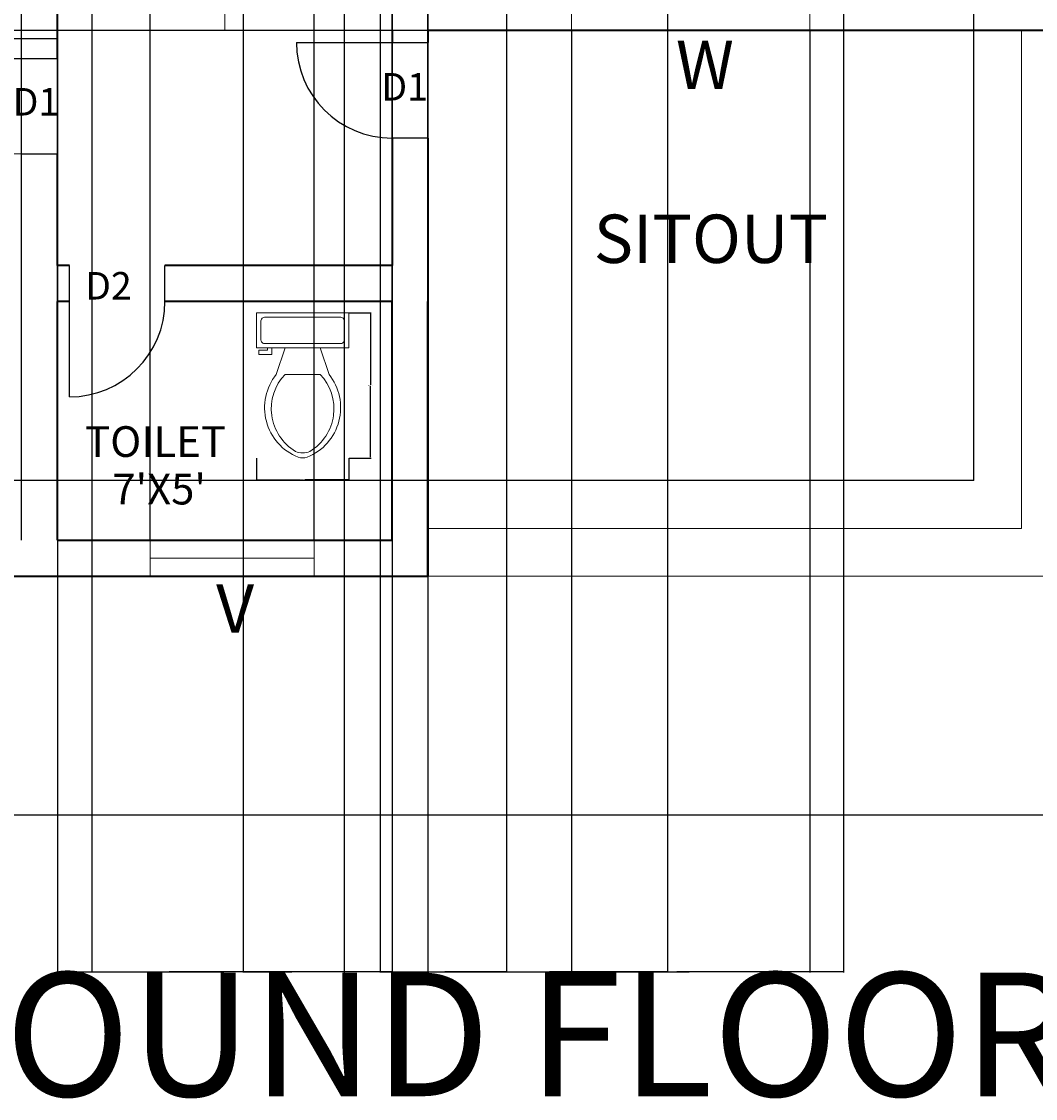
# Model space of a CAD drawing. Units: feet. Extents: x 2270 to 3094, y 1543 to 2352.
# Tile 2 of 6: x 2563 to 2817, y 1543 to 1813. Entities that reach past the tile are written whole.
import ezdxf

# ---------------------------------------------------------------- set-up
doc = ezdxf.new("R2010")
doc.units = ezdxf.units.FT
for name, color, linetype, lineweight in [('A-ANNO-DIMS', 2, 'Continuous', 18), ('A-ANNO-TEXT', 7, 'Continuous', 18), ('A-ANNO-TITL', 7, 'Continuous', 35), ('A-AREA-IDEN', 7, 'Continuous', 18), ('A-DOOR', 3, 'Continuous', 25), ('A-FLOR-FIXT', 8, 'Continuous', 18), ('A-FLOR-STRS', 7, 'Continuous', 18), ('A-GLAZ', 4, 'Continuous', 18), ('A-WALL', 7, 'Continuous', 35), ('C-PROP', 8, 'Continuous', 25)]:
    doc.layers.add(name, color=color, linetype=linetype, lineweight=lineweight)
doc.styles.get("Standard").update_dxf_attribs({"font": 'arial.ttf'})
doc.dimstyles.get("Standard").update_dxf_attribs({"dimtxt": 0.18, "dimasz": 0.18, "dimexe": 0.18, "dimexo": 0.0625, "dimgap": 0.09, "dimtad": 0, "dimtih": 1, "dimtoh": 1, "dimdec": 4, "dimzin": 0, "dimdsep": 46, "dimtxsty": 'Standard', "dimcen": 0.09, "dimadec": 0, "dimazin": 0, "dimtfac": 1, "dimtdec": 4, "dimtofl": 0, "dimtmove": 0, "dimatfit": 3, "dimfxl": 1, "dimtolj": 1, "dimtzin": 0, "dimarcsym": 0})

# ---------------------------------------------------------------- blocks, each defined once
blk = doc.blocks.new('Toilet - top')
for p, q in [((9.5, -6), (9.5, -2)), ((-10, -8.5), (-8, -8.5)), ((-10, -9.5), (-10, -8.5)), ((-7, -9.5), (-10, -9.5)), ((-8, -8.5), (-8, -8)), ((-7, -8), (-7, -9.5)), ((-4, -8), (-6, -14)), ((4, -8), (6, -14)), ((4, -14), (-4, -14))]:
    blk.add_line(p, q)
blk.add_lwpolyline([(10.5, -8), (10.5, 0), (-10.5, 0), (-10.5, -8)], close=True)
for points in [[(-9.5, -2), (-9.5, -6)], [(8.5, -1), (-8.5, -1)], [(-8.5, -7), (8.5, -7)]]:
    blk.add_lwpolyline(points)
for centre, radius, start, end in [((-8.62, -1.88), 0.884, 81.8699, 188.1301), ((8.62, -1.88), 0.884, 351.8699, 98.1301), ((-8.62, -6.12), 0.884, 171.8699, 278.1301), ((8.62, -6.12), 0.884, 261.8699, 8.1301), ((3.52, -21.58), 12.17, 141.4691, 247.9714), ((4.2, -21.82), 11.33, 136.3677, 238.9468), ((-3.52, -21.58), 12.17, 292.0284, 38.5307), ((-4.2, -21.82), 11.33, 301.053, 43.6321), ((0, -27.88), 4, 245.7318, 294.2682), ((0, -29), 4, 254.8605, 285.1395)]:
    blk.add_arc(centre, radius, start, end)
blk = doc.blocks.new('DOOR-SWING-24')
blk.add_line((33, 0), (0, 0))
blk.add_arc((9, 0), 24, 0, 90)
blk = doc.blocks.new('*D10')
at = {"layer": 'A-ANNO-DIMS', "color": 0, "lineweight": -2, "transparency": 16777216}
for p, q in [((2538.67, 1804.15), (2538.67, 1809.21)), ((2538.85, 1809.03), (2554.23, 1809.03)), ((2571.49, 1809.03), (2556.1, 1809.03)), ((2571.67, 1804.15), (2571.67, 1809.21))]:
    blk.add_line(p, q, dxfattribs=at)
at = {"layer": 'A-ANNO-DIMS', "color": 0, "transparency": 16777216}
for points in [[(2538.85, 1809.06), (2538.85, 1809), (2538.67, 1809.03)], [(2571.49, 1809.06), (2571.49, 1809), (2571.67, 1809.03)]]:
    blk.add_solid(points, dxfattribs=at)
at = {"layer": 'Defpoints', "color": 0, "transparency": 16777216}
for p in [(2538.67, 1809.03), (2538.67, 1804.08), (2571.67, 1804.08)]:
    blk.add_point(p, dxfattribs=at)
at = {"layer": 'A-ANNO-DIMS', "color": 0, "transparency": 16777216, "insert": (2555.17, 1809.03), "char_height": 0.18, "attachment_point": 5}
blk.add_mtext('\\A1;DOOR 33 TYP.', dxfattribs=at)
blk = doc.blocks.new('*D14')
at = {"layer": 'A-ANNO-DIMS', "color": 0, "lineweight": -2, "transparency": 16777216}
for p, q in [((2644.87, 1740.2), (2650.46, 1740.2)), ((2650.28, 1740.02), (2650.28, 1722.15)), ((2650.28, 1703.92), (2650.28, 1721.79)), ((2644.87, 1703.74), (2650.46, 1703.74))]:
    blk.add_line(p, q, dxfattribs=at)
at = {"layer": 'A-ANNO-DIMS', "color": 0, "transparency": 16777216}
for points in [[(2650.25, 1740.02), (2650.31, 1740.02), (2650.28, 1740.2)], [(2650.25, 1703.92), (2650.31, 1703.92), (2650.28, 1703.74)]]:
    blk.add_solid(points, dxfattribs=at)
at = {"layer": 'Defpoints', "color": 0, "transparency": 16777216}
for p in [(2644.81, 1740.2), (2650.28, 1740.2), (2644.81, 1703.74)]:
    blk.add_point(p, dxfattribs=at)
at = {"layer": 'A-ANNO-DIMS', "color": 0, "transparency": 16777216, "insert": (2650.28, 1721.97), "char_height": 0.18, "attachment_point": 5}
blk.add_mtext('\\A1;WC 36 TYP.', dxfattribs=at)
blk = doc.blocks.new('*D15')
at = {"layer": 'A-ANNO-DIMS', "color": 0, "lineweight": -2, "transparency": 16777216}
for p, q in [((2621.64, 1703.68), (2621.64, 1698.09)), ((2644.81, 1703.68), (2644.81, 1698.09)), ((2621.82, 1698.27), (2632.7, 1698.27)), ((2644.63, 1698.27), (2633.75, 1698.27))]:
    blk.add_line(p, q, dxfattribs=at)
at = {"layer": 'A-ANNO-DIMS', "color": 0, "transparency": 16777216}
for points in [[(2621.82, 1698.3), (2621.82, 1698.24), (2621.64, 1698.27)], [(2644.63, 1698.3), (2644.63, 1698.24), (2644.81, 1698.27)]]:
    blk.add_solid(points, dxfattribs=at)
at = {"layer": 'Defpoints', "color": 0, "transparency": 16777216}
for p in [(2621.64, 1703.74), (2644.81, 1703.74), (2644.81, 1698.27)]:
    blk.add_point(p, dxfattribs=at)
at = {"layer": 'A-ANNO-DIMS', "color": 0, "transparency": 16777216, "insert": (2633.23, 1698.27), "char_height": 0.18, "attachment_point": 5}
blk.add_mtext('\\A1;23 TYP.', dxfattribs=at)
blk = doc.blocks.new('*D34')
at = {"layer": 'A-ANNO-DIMS', "color": 0, "lineweight": -2, "transparency": 16777216}
for p, q in [((2580.32, 2252.02), (2580.32, 1574.6)), ((2618.3, 2252.02), (2618.3, 1574.6)), ((2580.5, 1574.78), (2598.92, 1574.78)), ((2618.12, 1574.78), (2599.7, 1574.78))]:
    blk.add_line(p, q, dxfattribs=at)
at = {"layer": 'A-ANNO-DIMS', "color": 0, "transparency": 16777216}
for points in [[(2580.5, 1574.81), (2580.5, 1574.75), (2580.32, 1574.78)], [(2618.12, 1574.81), (2618.12, 1574.75), (2618.3, 1574.78)]]:
    blk.add_solid(points, dxfattribs=at)
at = {"layer": 'Defpoints', "color": 0, "transparency": 16777216}
for p in [(2580.32, 2252.08), (2618.3, 2252.08), (2618.3, 1574.78)]:
    blk.add_point(p, dxfattribs=at)
at = {"layer": 'A-ANNO-DIMS', "color": 0, "transparency": 16777216, "insert": (2599.31, 1574.78), "char_height": 0.18, "attachment_point": 5}
blk.add_mtext('\\A1;37.98', dxfattribs=at)
blk = doc.blocks.new('*D35')
at = {"layer": 'A-ANNO-DIMS', "color": 0, "lineweight": -2, "transparency": 16777216}
for p, q in [((2618.3, 2243.02), (2618.3, 1574.6)), ((2643.67, 2243.02), (2643.67, 1574.6)), ((2618.48, 1574.78), (2630.52, 1574.78)), ((2643.49, 1574.78), (2631.45, 1574.78))]:
    blk.add_line(p, q, dxfattribs=at)
at = {"layer": 'A-ANNO-DIMS', "color": 0, "transparency": 16777216}
for points in [[(2618.48, 1574.81), (2618.48, 1574.75), (2618.3, 1574.78)], [(2643.49, 1574.81), (2643.49, 1574.75), (2643.67, 1574.78)]]:
    blk.add_solid(points, dxfattribs=at)
at = {"layer": 'Defpoints', "color": 0, "transparency": 16777216}
for p in [(2618.3, 2243.08), (2643.67, 2243.08), (2643.67, 1574.78)]:
    blk.add_point(p, dxfattribs=at)
at = {"layer": 'A-ANNO-DIMS', "color": 0, "transparency": 16777216, "insert": (2630.98, 1574.78), "char_height": 0.18, "attachment_point": 5}
blk.add_mtext('\\A1;25.366', dxfattribs=at)
blk = doc.blocks.new('*D36')
at = {"layer": 'A-ANNO-DIMS', "color": 0, "lineweight": -2, "transparency": 16777216}
for p, q in [((2652.67, 2243.02), (2652.67, 1574.6)), ((2684.42, 2243.02), (2684.42, 1574.6)), ((2652.85, 1574.78), (2668.15, 1574.78)), ((2684.24, 1574.78), (2668.94, 1574.78))]:
    blk.add_line(p, q, dxfattribs=at)
at = {"layer": 'A-ANNO-DIMS', "color": 0, "transparency": 16777216}
for points in [[(2652.85, 1574.81), (2652.85, 1574.75), (2652.67, 1574.78)], [(2684.24, 1574.81), (2684.24, 1574.75), (2684.42, 1574.78)]]:
    blk.add_solid(points, dxfattribs=at)
at = {"layer": 'Defpoints', "color": 0, "transparency": 16777216}
for p in [(2652.67, 2243.08), (2684.42, 2243.08), (2684.42, 1574.78)]:
    blk.add_point(p, dxfattribs=at)
at = {"layer": 'A-ANNO-DIMS', "color": 0, "transparency": 16777216, "insert": (2668.55, 1574.78), "char_height": 0.18, "attachment_point": 5}
blk.add_mtext('\\A1;31.76', dxfattribs=at)
blk = doc.blocks.new('*D37')
at = {"layer": 'A-ANNO-DIMS', "color": 0, "lineweight": -2, "transparency": 16777216}
for p, q in [((2684.42, 2243.02), (2684.42, 1574.6)), ((2769.01, 2243.02), (2769.01, 1574.6)), ((2684.6, 1574.78), (2726.32, 1574.78)), ((2768.83, 1574.78), (2727.11, 1574.78))]:
    blk.add_line(p, q, dxfattribs=at)
at = {"layer": 'A-ANNO-DIMS', "color": 0, "transparency": 16777216}
for points in [[(2684.6, 1574.81), (2684.6, 1574.75), (2684.42, 1574.78)], [(2768.83, 1574.81), (2768.83, 1574.75), (2769.01, 1574.78)]]:
    blk.add_solid(points, dxfattribs=at)
at = {"layer": 'Defpoints', "color": 0, "transparency": 16777216}
for p in [(2684.42, 2243.08), (2769.01, 2243.08), (2769.01, 1574.78)]:
    blk.add_point(p, dxfattribs=at)
at = {"layer": 'A-ANNO-DIMS', "color": 0, "transparency": 16777216, "insert": (2726.71, 1574.78), "char_height": 0.18, "attachment_point": 5}
blk.add_mtext('\\A1;84.58', dxfattribs=at)
blk = doc.blocks.new('*D46')
at = {"layer": 'A-ANNO-DIMS', "color": 0, "lineweight": -2, "transparency": 16777216}
for p, q in [((2700.7, 1811.02), (2700.7, 1574.6)), ((2760.54, 1811.02), (2760.54, 1574.6)), ((2700.88, 1574.78), (2730.23, 1574.78)), ((2760.36, 1574.78), (2731.01, 1574.78))]:
    blk.add_line(p, q, dxfattribs=at)
at = {"layer": 'A-ANNO-DIMS', "color": 0, "transparency": 16777216}
for points in [[(2700.88, 1574.81), (2700.88, 1574.75), (2700.7, 1574.78)], [(2760.36, 1574.81), (2760.36, 1574.75), (2760.54, 1574.78)]]:
    blk.add_solid(points, dxfattribs=at)
at = {"layer": 'Defpoints', "color": 0, "transparency": 16777216}
for p in [(2700.7, 1811.08), (2760.54, 1811.08), (2760.54, 1574.78)]:
    blk.add_point(p, dxfattribs=at)
at = {"layer": 'A-ANNO-DIMS', "color": 0, "transparency": 16777216, "insert": (2730.62, 1574.78), "char_height": 0.18, "attachment_point": 5}
blk.add_mtext('\\A1;59.83', dxfattribs=at)
blk = doc.blocks.new('*D48')
at = {"layer": 'A-ANNO-DIMS', "color": 0, "lineweight": -2, "transparency": 16777216}
for p, q in [((2664.67, 1698.15), (2664.67, 2351.56)), ((2664.85, 2351.38), (2732.89, 2351.38)), ((2801.49, 2351.38), (2733.45, 2351.38)), ((2801.67, 1698.15), (2801.67, 2351.56))]:
    blk.add_line(p, q, dxfattribs=at)
at = {"layer": 'A-ANNO-DIMS', "color": 0, "transparency": 16777216}
for points in [[(2664.85, 2351.41), (2664.85, 2351.35), (2664.67, 2351.38)], [(2801.49, 2351.41), (2801.49, 2351.35), (2801.67, 2351.38)]]:
    blk.add_solid(points, dxfattribs=at)
at = {"layer": 'Defpoints', "color": 0, "transparency": 16777216}
for p in [(2801.67, 2351.38), (2664.67, 1698.08), (2801.67, 1698.08)]:
    blk.add_point(p, dxfattribs=at)
at = {"layer": 'A-ANNO-DIMS', "color": 0, "transparency": 16777216, "insert": (2733.17, 2351.38), "char_height": 0.18, "attachment_point": 5}
blk.add_mtext('\\A1;137', dxfattribs=at)
blk = doc.blocks.new('*D49')
at = {"layer": 'A-ANNO-DIMS', "color": 0, "lineweight": -2, "transparency": 16777216}
for p, q in [((2801.6, 1811.08), (2270.19, 1811.08)), ((2270.37, 1810.9), (2270.37, 1754.77)), ((2270.37, 1698.26), (2270.37, 1754.4)), ((2801.6, 1698.08), (2270.19, 1698.08))]:
    blk.add_line(p, q, dxfattribs=at)
at = {"layer": 'A-ANNO-DIMS', "color": 0, "transparency": 16777216}
for points in [[(2270.34, 1810.9), (2270.4, 1810.9), (2270.37, 1811.08)], [(2270.34, 1698.26), (2270.4, 1698.26), (2270.37, 1698.08)]]:
    blk.add_solid(points, dxfattribs=at)
at = {"layer": 'Defpoints', "color": 0, "transparency": 16777216}
for p in [(2270.37, 1811.08), (2801.67, 1811.08), (2801.67, 1698.08)]:
    blk.add_point(p, dxfattribs=at)
at = {"layer": 'A-ANNO-DIMS', "color": 0, "transparency": 16777216, "insert": (2270.37, 1754.58), "char_height": 0.18, "attachment_point": 5}
blk.add_mtext('\\A1;113', dxfattribs=at)
blk = doc.blocks.new('*D52')
at = {"layer": 'A-ANNO-DIMS', "color": 0, "lineweight": -2, "transparency": 16777216}
for p, q in [((2594.98, 1683.15), (2594.98, 2351.56)), ((2595.16, 2351.38), (2615.09, 2351.38)), ((2635.97, 2351.38), (2616.03, 2351.38)), ((2636.15, 1683.15), (2636.15, 2351.56))]:
    blk.add_line(p, q, dxfattribs=at)
at = {"layer": 'A-ANNO-DIMS', "color": 0, "transparency": 16777216}
for points in [[(2595.16, 2351.41), (2595.16, 2351.35), (2594.98, 2351.38)], [(2635.97, 2351.41), (2635.97, 2351.35), (2636.15, 2351.38)]]:
    blk.add_solid(points, dxfattribs=at)
at = {"layer": 'Defpoints', "color": 0, "transparency": 16777216}
for p in [(2636.15, 2351.38), (2594.98, 1683.08), (2636.15, 1683.08)]:
    blk.add_point(p, dxfattribs=at)
at = {"layer": 'A-ANNO-DIMS', "color": 0, "transparency": 16777216, "insert": (2615.56, 2351.38), "char_height": 0.18, "attachment_point": 5}
blk.add_mtext('\\A1;41.175', dxfattribs=at)
blk = doc.blocks.new('*D53')
at = {"layer": 'A-ANNO-DIMS', "color": 0, "lineweight": -2, "transparency": 16777216}
for p, q in [((2636.15, 1683.15), (2636.15, 2351.56)), ((2636.33, 2351.38), (2645.45, 2351.38)), ((2655.49, 2351.38), (2646.36, 2351.38)), ((2655.67, 1683.15), (2655.67, 2351.56))]:
    blk.add_line(p, q, dxfattribs=at)
at = {"layer": 'A-ANNO-DIMS', "color": 0, "transparency": 16777216}
for points in [[(2636.33, 2351.41), (2636.33, 2351.35), (2636.15, 2351.38)], [(2655.49, 2351.41), (2655.49, 2351.35), (2655.67, 2351.38)]]:
    blk.add_solid(points, dxfattribs=at)
at = {"layer": 'Defpoints', "color": 0, "transparency": 16777216}
for p in [(2655.67, 2351.38), (2636.15, 1683.08), (2655.67, 1683.08)]:
    blk.add_point(p, dxfattribs=at)
at = {"layer": 'A-ANNO-DIMS', "color": 0, "transparency": 16777216, "insert": (2645.91, 2351.38), "char_height": 0.18, "attachment_point": 5}
blk.add_mtext('\\A1;19.516', dxfattribs=at)
blk = doc.blocks.new('*D61')
at = {"layer": 'A-ANNO-DIMS', "color": 0, "lineweight": -2, "transparency": 16777216}
for p, q in [((2571.67, 1968.02), (2571.67, 1574.6)), ((2655.67, 1968.02), (2655.67, 1574.6)), ((2571.85, 1574.78), (2613.45, 1574.78)), ((2655.49, 1574.78), (2613.88, 1574.78))]:
    blk.add_line(p, q, dxfattribs=at)
at = {"layer": 'A-ANNO-DIMS', "color": 0, "transparency": 16777216}
for points in [[(2571.85, 1574.81), (2571.85, 1574.75), (2571.67, 1574.78)], [(2655.49, 1574.81), (2655.49, 1574.75), (2655.67, 1574.78)]]:
    blk.add_solid(points, dxfattribs=at)
at = {"layer": 'Defpoints', "color": 0, "transparency": 16777216}
for p in [(2571.67, 1968.08), (2655.67, 1968.08), (2655.67, 1574.78)]:
    blk.add_point(p, dxfattribs=at)
at = {"layer": 'A-ANNO-DIMS', "color": 0, "transparency": 16777216, "insert": (2613.67, 1574.78), "char_height": 0.18, "attachment_point": 5}
blk.add_mtext('\\A1;84', dxfattribs=at)
blk = doc.blocks.new('*D65')
at = {"layer": 'A-ANNO-DIMS', "color": 0, "lineweight": -2, "transparency": 16777216}
for p, q in [((2562.67, 1683.15), (2562.67, 2351.56)), ((2562.85, 2351.38), (2567.02, 2351.38)), ((2571.49, 2351.38), (2567.32, 2351.38)), ((2571.67, 1683.15), (2571.67, 2351.56))]:
    blk.add_line(p, q, dxfattribs=at)
at = {"layer": 'A-ANNO-DIMS', "color": 0, "transparency": 16777216}
for points in [[(2562.85, 2351.41), (2562.85, 2351.35), (2562.67, 2351.38)], [(2571.49, 2351.41), (2571.49, 2351.35), (2571.67, 2351.38)]]:
    blk.add_solid(points, dxfattribs=at)
at = {"layer": 'Defpoints', "color": 0, "transparency": 16777216}
for p in [(2571.67, 2351.38), (2562.67, 1683.08), (2571.67, 1683.08)]:
    blk.add_point(p, dxfattribs=at)
at = {"layer": 'A-ANNO-DIMS', "color": 0, "transparency": 16777216, "insert": (2567.17, 2351.38), "char_height": 0.18, "attachment_point": 5}
blk.add_mtext('\\A1;9', dxfattribs=at)
blk = doc.blocks.new('*D67')
at = {"layer": 'A-ANNO-DIMS', "color": 0, "lineweight": -2, "transparency": 16777216}
for p, q in [((2664.67, 1968.02), (2664.67, 1574.6)), ((2724.84, 1968.02), (2724.84, 1574.6)), ((2664.85, 1574.78), (2694.36, 1574.78)), ((2724.66, 1574.78), (2695.15, 1574.78))]:
    blk.add_line(p, q, dxfattribs=at)
at = {"layer": 'A-ANNO-DIMS', "color": 0, "transparency": 16777216}
for points in [[(2664.85, 1574.81), (2664.85, 1574.75), (2664.67, 1574.78)], [(2724.66, 1574.81), (2724.66, 1574.75), (2724.84, 1574.78)]]:
    blk.add_solid(points, dxfattribs=at)
at = {"layer": 'Defpoints', "color": 0, "transparency": 16777216}
for p in [(2664.67, 1968.08), (2724.84, 1968.08), (2664.67, 1574.78)]:
    blk.add_point(p, dxfattribs=at)
at = {"layer": 'A-ANNO-DIMS', "color": 0, "transparency": 16777216, "insert": (2694.75, 1574.78), "char_height": 0.18, "attachment_point": 5}
blk.add_mtext('\\A1;60.17', dxfattribs=at)

msp = doc.modelspace()

# ---------------------------------------------------------------- linework, layer by layer
at = {"layer": 'A-DOOR'}
for p, q in [((2664.6659, 1784.0845), (2655.6659, 1784.0845)), ((2562.6659, 1780.0845), (2571.6659, 1780.0845)), ((2598.6659, 1743.0845), (2598.6659, 1752.0845))]:
    msp.add_line(p, q, dxfattribs=at)
at = {"layer": 'A-FLOR-STRS'}
for p, q in [((2613.6659, 1811.0845), (2613.6659, 1968.0845)), ((2655.6659, 1811.0845), (2613.6659, 1811.0845))]:
    msp.add_line(p, q, dxfattribs=at)
for points in [[(2825.6659, 1811.0845), (2825.6659, 1674.0845), (2664.6659, 1674.0845)], [(2813.6659, 1811.0845), (2813.6659, 1686.0845), (2664.6659, 1686.0845)], [(2801.6659, 1811.0845), (2801.6659, 1698.0845), (2664.6659, 1698.0845)]]:
    msp.add_lwpolyline(points, dxfattribs=at)
at = {"layer": 'A-GLAZ'}
for p, q in [((2700.7017, 1820.0845), (2700.7017, 1811.0845)), ((2760.5365, 1820.0845), (2760.5365, 1811.0845)), ((2594.9751, 1683.0845), (2594.9751, 1674.0845)), ((2636.1502, 1683.0845), (2636.1502, 1674.0845)), ((2594.9751, 1678.5845), (2636.1502, 1678.5845))]:
    msp.add_line(p, q, dxfattribs=at)
at = {"layer": 'A-WALL'}
for p, q in [((2571.6659, 1804.0845), (2571.6659, 1968.0845)), ((2655.6659, 1811.0845), (2655.6659, 1808.0845)), ((2825.6659, 1811.0845), (2664.6659, 1811.0845)), ((2664.6659, 1811.0845), (2664.6659, 1808.0845)), ((2571.6659, 1804.0845), (2571.6659, 1807.0845)), ((2655.6659, 1784.0845), (2655.6659, 1752.0845)), ((2664.6659, 1784.0845), (2664.6659, 1674.0845)), ((2571.6659, 1752.0845), (2571.6659, 1780.0845)), ((2571.6659, 1752.0845), (2571.6659, 1780.0845)), ((2574.6659, 1752.0845), (2571.6659, 1752.0845)), ((2655.6659, 1752.0845), (2598.6659, 1752.0845)), ((2571.6659, 1683.0845), (2571.6659, 1743.0845)), ((2574.6659, 1743.0845), (2571.6659, 1743.0845)), ((2655.6659, 1743.0845), (2598.6659, 1743.0845)), ((2655.6659, 1683.0845), (2655.6659, 1743.0845)), ((2664.6659, 1674.0845), (2664.6659, 1743.0845)), ((2571.6659, 1683.0845), (2655.6659, 1683.0845)), ((2369.6659, 1674.0845), (2664.6659, 1674.0845)), ((2571.6659, 1674.0845), (2664.6659, 1674.0845))]:
    msp.add_line(p, q, dxfattribs=at)
at = {"layer": 'C-PROP'}
msp.add_line((3054.6659, 1614.0845), (2309.6659, 1614.0845), dxfattribs=at)

# ---------------------------------------------------------------- block references
at = {"layer": 'A-DOOR'}
for p, rotation in [((2664.6658, 1808.084), 180), ((2571.6658, 1804.084), 180), ((2574.6664, 1752.0844), 269.9999999999994)]:
    msp.add_blockref('DOOR-SWING-24', p, dxfattribs=dict(at, rotation=rotation))
at = {"layer": 'A-FLOR-FIXT', "xscale": 1.103431246609896, "yscale": 1.103431246609896, "zscale": 1.103431246609896}
msp.add_blockref('Toilet - top', (2633.225, 1740.2029), dxfattribs=at)

# ---------------------------------------------------------------- texts
at = {"layer": 'A-ANNO-TEXT'}
for s, height, p in [('W', 12.1456, (2726.9297, 1796.3556)), ('D1', 6.89564, (2652.9851, 1793.5047)), ('D1', 6.89564, (2560.4382, 1789.7406)), ('D2', 6.89564, (2578.6351, 1743.5412)), ('V', 12.1456, (2611.5026, 1659.8775))]:
    msp.add_text(s, height=height, dxfattribs=at).set_placement(p)
at = {"layer": 'A-ANNO-TITL'}
msp.add_text('GROUND FLOOR', height=31.058177, dxfattribs=at).set_placement((2502.4393, 1543.4965))
at = {"layer": 'A-AREA-IDEN'}
for s, height, p in [('SITOUT', 12.14556, (2706.2935, 1752.7121)), ('TOILET', 7.69843, (2578.6377, 1704.0282)), ("7'X5'", 7.69843, (2585.4516, 1692.0804))]:
    msp.add_text(s, height=height, dxfattribs=at).set_placement(p)

# ---------------------------------------------------------------- dimensions: what is measured, and where the dimension line sits
at = {"layer": 'A-ANNO-DIMS'}
for base, p1, p2, override, picture, middle in [((2571.6659, 2351.3845), (2562.6659, 1683.0845), (2571.6659, 1683.0845), {"dimdec": 0, "dimlfac": 1, "dimrnd": 0, "dimzin": 0, "dimdsep": 46, "dimlunit": 2}, '*D65', (2567.1659, 2351.3845)), ((2636.1502, 2351.3845), (2594.9751, 1683.0845), (2636.1502, 1683.0845), {"dimdec": 3, "dimlfac": 1, "dimrnd": 0, "dimzin": 0, "dimdsep": 46, "dimlunit": 2}, '*D52', (2615.5626, 2351.3845)), ((2655.6659, 2351.3845), (2636.1502, 1683.0845), (2655.6659, 1683.0845), {"dimdec": 3, "dimlfac": 1, "dimrnd": 0, "dimzin": 0, "dimdsep": 46, "dimlunit": 2}, '*D53', (2645.9081, 2351.3845)), ((2801.6659, 2351.3845), (2664.6659, 1698.0845), (2801.6659, 1698.0845), {"dimdec": 0, "dimlfac": 1, "dimrnd": 0, "dimzin": 0, "dimdsep": 46, "dimlunit": 2}, '*D48', (2733.1659, 2351.3845)), ((2618.2997, 1574.7845), (2580.3205, 2252.0845), (2618.2997, 2252.0845), {"dimdec": 2, "dimlfac": 1, "dimrnd": 0, "dimzin": 0, "dimdsep": 46, "dimlunit": 2}, '*D34', (2599.3101, 1574.7845)), ((2643.6659, 1574.7845), (2618.2997, 2243.0845), (2643.6659, 2243.0845), {"dimdec": 3, "dimlfac": 1, "dimrnd": 0, "dimzin": 0, "dimdsep": 46, "dimlunit": 2}, '*D35', (2630.9828, 1574.7845)), ((2684.4243, 1574.7845), (2652.6659, 2243.0845), (2684.4243, 2243.0845), {"dimdec": 2, "dimlfac": 1, "dimrnd": 0, "dimzin": 0, "dimdsep": 46, "dimlunit": 2}, '*D36', (2668.5451, 1574.7845)), ((2769.0053, 1574.7845), (2684.4243, 2243.0845), (2769.0053, 2243.0845), {"dimdec": 2, "dimlfac": 1, "dimrnd": 0, "dimzin": 0, "dimdsep": 46, "dimlunit": 2}, '*D37', (2726.7148, 1574.7845)), ((2655.6659, 1574.7845), (2571.6659, 1968.0845), (2655.6659, 1968.0845), {"dimdec": 0, "dimlfac": 1, "dimrnd": 0, "dimzin": 0, "dimdsep": 46, "dimlunit": 2}, '*D61', (2613.6659, 1574.7845)), ((2664.6659, 1574.7845), (2724.8399, 1968.0845), (2664.6659, 1968.0845), {"dimdec": 2, "dimlfac": 1, "dimrnd": 0, "dimzin": 0, "dimdsep": 46, "dimlunit": 2}, '*D67', (2694.7529, 1574.7845)), ((2760.5365, 1574.7845), (2700.7017, 1811.0845), (2760.5365, 1811.0845), {"dimdec": 2, "dimlfac": 1, "dimrnd": 0, "dimzin": 0, "dimdsep": 46, "dimlunit": 2}, '*D46', (2730.6191, 1574.7845))]:
    dim = msp.add_linear_dim(base=base, p1=p1, p2=p2, dimstyle='Standard', override=override, dxfattribs=at)
    dim.commit()
    dim.dimension.update_dxf_attribs({"geometry": picture, "text_midpoint": middle})
dim = msp.add_linear_dim(base=(2270.3659, 1811.0845), p1=(2801.6659, 1698.0845), p2=(2801.6659, 1811.0845), angle=90, dimstyle='Standard', override={"dimdec": 0, "dimlfac": 1, "dimrnd": 0, "dimzin": 0, "dimdsep": 46, "dimlunit": 2}, dxfattribs=at)
dim.commit()
dim.dimension.update_dxf_attribs({"geometry": '*D49', "text_midpoint": (2270.3659, 1754.5845)})
for base, p1, p2, angle, text, picture, middle in [((2538.6659, 1809.0345), (2571.6659, 1804.0845), (2538.6659, 1804.0845), 180, 'DOOR <> TYP.', '*D10', (2555.1659, 1809.0345)), ((2650.2807, 1740.2029), (2644.8111, 1703.7387), (2644.8111, 1740.2029), 90, 'WC <> TYP.', '*D14', (2650.2807, 1721.9708))]:
    dim = msp.add_linear_dim(base=base, p1=p1, p2=p2, angle=angle, text=text, dimstyle='Standard', override={"dimdec": 0, "dimlfac": 1, "dimrnd": 0, "dimzin": 0, "dimdsep": 46, "dimlunit": 2}, dxfattribs=at)
    dim.commit()
    dim.dimension.update_dxf_attribs({"geometry": picture, "text_midpoint": middle})
dim = msp.add_linear_dim(base=(2644.8111, 1698.269), p1=(2621.639, 1703.7387), p2=(2644.8111, 1703.7387), text='<> TYP.', dimstyle='Standard', override={"dimdec": 0, "dimlfac": 1, "dimrnd": 0, "dimzin": 0, "dimdsep": 46, "dimlunit": 2}, dxfattribs=at)
dim.commit()
dim.dimension.update_dxf_attribs({"geometry": '*D15', "text_midpoint": (2633.225, 1698.269)})

doc.saveas('drawing.dxf')
